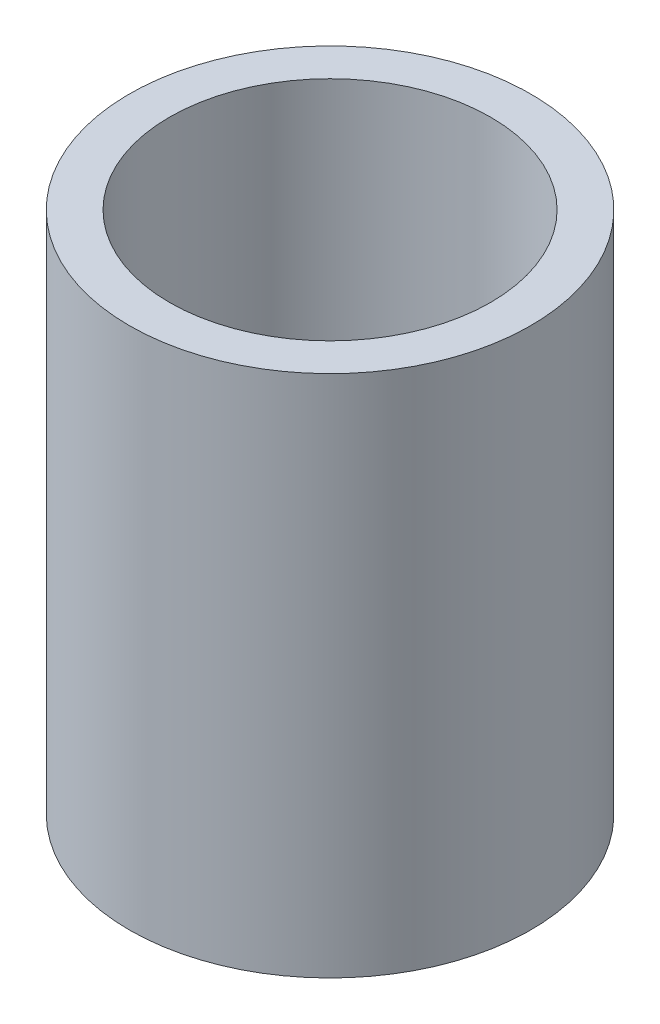
ISO-10303-21;
HEADER;
FILE_DESCRIPTION(('STEP AP214'),'2;1');
FILE_NAME('part.step','',(''),(''),'','','');
FILE_SCHEMA(('AUTOMOTIVE_DESIGN { 1 0 10303 214 1 1 1 1 }'));
ENDSEC;
DATA;
#1=APPLICATION_CONTEXT('core data for automotive mechanical design processes');
#2=APPLICATION_PROTOCOL_DEFINITION('international standard','automotive_design',2000,#1);
#3=PRODUCT_CONTEXT('',#1,'mechanical');
#4=PRODUCT('Part','Part','',(#3));
#5=PRODUCT_RELATED_PRODUCT_CATEGORY('part','',(#4));
#6=PRODUCT_DEFINITION_FORMATION('','',#4);
#7=PRODUCT_DEFINITION_CONTEXT('part definition',#1,'design');
#8=PRODUCT_DEFINITION('design','',#6,#7);
#9=PRODUCT_DEFINITION_SHAPE('','',#8);
#10=(LENGTH_UNIT() NAMED_UNIT(*) SI_UNIT(.MILLI.,.METRE.));
#11=(NAMED_UNIT(*) PLANE_ANGLE_UNIT() SI_UNIT($,.RADIAN.));
#12=(NAMED_UNIT(*) SI_UNIT($,.STERADIAN.) SOLID_ANGLE_UNIT());
#13=UNCERTAINTY_MEASURE_WITH_UNIT(LENGTH_MEASURE(1.E-05),#10,'distance_accuracy_value','');
#14=(GEOMETRIC_REPRESENTATION_CONTEXT(3) GLOBAL_UNCERTAINTY_ASSIGNED_CONTEXT((#13)) GLOBAL_UNIT_ASSIGNED_CONTEXT((#10,
#11,#12)) REPRESENTATION_CONTEXT('',''));
#15=CARTESIAN_POINT('',(0.,0.,0.));
#16=DIRECTION('',(0.,0.,1.));
#17=DIRECTION('',(1.,0.,0.));
#18=AXIS2_PLACEMENT_3D('',#15,#16,#17);
#19=CARTESIAN_POINT('',(0.,81.5,0.));
#20=DIRECTION('',(0.,1.,0.));
#21=DIRECTION('',(0.,0.,1.));
#22=AXIS2_PLACEMENT_3D('',#19,#20,#21);
#23=PLANE('',#22);
#24=CARTESIAN_POINT('',(0.,81.5,0.));
#25=DIRECTION('',(0.,1.,0.));
#26=DIRECTION('',(0.,0.,1.));
#27=AXIS2_PLACEMENT_3D('',#24,#25,#26);
#28=CIRCLE('',#27,62.5);
#29=CARTESIAN_POINT('',(0.,81.5,62.5));
#30=VERTEX_POINT('',#29);
#31=EDGE_CURVE('E10',#30,#30,#28,.T.);
#32=ORIENTED_EDGE('',*,*,#31,.T.);
#33=EDGE_LOOP('',(#32));
#34=FACE_BOUND('',#33,.T.);
#35=CARTESIAN_POINT('',(0.,81.5,0.));
#36=DIRECTION('',(0.,1.,0.));
#37=DIRECTION('',(0.,0.,1.));
#38=AXIS2_PLACEMENT_3D('',#35,#36,#37);
#39=CIRCLE('',#38,50.);
#40=CARTESIAN_POINT('',(0.,81.5,50.));
#41=VERTEX_POINT('',#40);
#42=EDGE_CURVE('E48',#41,#41,#39,.T.);
#43=ORIENTED_EDGE('',*,*,#42,.F.);
#44=EDGE_LOOP('',(#43));
#45=FACE_BOUND('',#44,.T.);
#46=ADVANCED_FACE('F40',(#34,#45),#23,.T.);
#47=CARTESIAN_POINT('',(0.,-81.5,0.));
#48=DIRECTION('',(0.,1.,0.));
#49=DIRECTION('',(0.,0.,1.));
#50=AXIS2_PLACEMENT_3D('',#47,#48,#49);
#51=PLANE('',#50);
#52=CARTESIAN_POINT('',(0.,-81.5,0.));
#53=DIRECTION('',(0.,1.,0.));
#54=DIRECTION('',(0.,0.,1.));
#55=AXIS2_PLACEMENT_3D('',#52,#53,#54);
#56=CIRCLE('',#55,62.5);
#57=CARTESIAN_POINT('',(0.,-81.5,62.5));
#58=VERTEX_POINT('',#57);
#59=EDGE_CURVE('E41',#58,#58,#56,.T.);
#60=ORIENTED_EDGE('',*,*,#59,.F.);
#61=EDGE_LOOP('',(#60));
#62=FACE_BOUND('',#61,.T.);
#63=CARTESIAN_POINT('',(0.,-81.5,0.));
#64=DIRECTION('',(0.,1.,0.));
#65=DIRECTION('',(0.,0.,1.));
#66=AXIS2_PLACEMENT_3D('',#63,#64,#65);
#67=CIRCLE('',#66,50.);
#68=CARTESIAN_POINT('',(0.,-81.5,50.));
#69=VERTEX_POINT('',#68);
#70=EDGE_CURVE('E49',#69,#69,#67,.T.);
#71=ORIENTED_EDGE('',*,*,#70,.T.);
#72=EDGE_LOOP('',(#71));
#73=FACE_BOUND('',#72,.T.);
#74=ADVANCED_FACE('F58',(#62,#73),#51,.F.);
#75=CARTESIAN_POINT('',(0.,81.5,0.));
#76=DIRECTION('',(0.,-1.,0.));
#77=DIRECTION('',(0.,0.,-1.));
#78=AXIS2_PLACEMENT_3D('',#75,#76,#77);
#79=CYLINDRICAL_SURFACE('',#78,62.5);
#80=ORIENTED_EDGE('',*,*,#31,.F.);
#81=EDGE_LOOP('',(#80));
#82=FACE_BOUND('',#81,.T.);
#83=ORIENTED_EDGE('',*,*,#59,.T.);
#84=EDGE_LOOP('',(#83));
#85=FACE_BOUND('',#84,.T.);
#86=ADVANCED_FACE('F39',(#82,#85),#79,.T.);
#87=CARTESIAN_POINT('',(0.,81.5,0.));
#88=DIRECTION('',(0.,-1.,0.));
#89=DIRECTION('',(0.,0.,-1.));
#90=AXIS2_PLACEMENT_3D('',#87,#88,#89);
#91=CYLINDRICAL_SURFACE('',#90,50.);
#92=ORIENTED_EDGE('',*,*,#42,.T.);
#93=EDGE_LOOP('',(#92));
#94=FACE_BOUND('',#93,.T.);
#95=ORIENTED_EDGE('',*,*,#70,.F.);
#96=EDGE_LOOP('',(#95));
#97=FACE_BOUND('',#96,.T.);
#98=ADVANCED_FACE('F57',(#94,#97),#91,.F.);
#99=CLOSED_SHELL('',(#46,#74,#86,#98));
#100=MANIFOLD_SOLID_BREP('B2',#99);
#101=ADVANCED_BREP_SHAPE_REPRESENTATION('',(#18,#100),#14);
#102=SHAPE_DEFINITION_REPRESENTATION(#9,#101);
ENDSEC;
END-ISO-10303-21;
